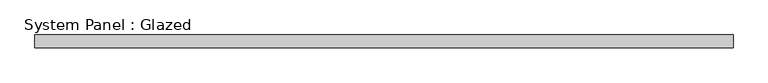
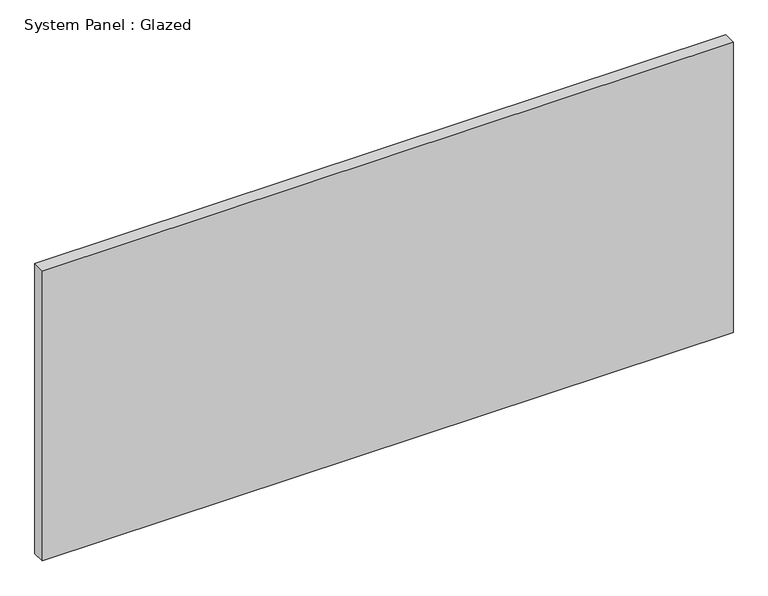
"""IFC4 building model written with IfcOpenShell, lengths in millimetres: plate geometry, System Panel : Glazed."""

from ifc_helpers import new_model, si_unit, origin, origin_with_axes, place, context, project, spatial, polyline, outline, extrude, source, transform, mapped, element, save


def system_panel_glazed_dff4d0e6(model_context):
    return source(origin(), model_context, "Body", "SweptSolid", [
        extrude(outline(polyline([(675.0, -49.5), (-675.0, -49.5), (-675.0, -24.5), (675.0, -24.5), (675.0, -49.5)])), origin_with_axes(), (0.0, 0.0, 1.0), 600.0),
    ])


if __name__ == "__main__":
    model = new_model("IFC4")
    model_context = context("Model", 3, world=origin())
    ifc_project = project(units=[si_unit("LENGTHUNIT", "METRE", prefix="MILLI")], contexts=[model_context])
    site = spatial("IfcSite", under=ifc_project)
    building = spatial("IfcBuilding", under=site)
    placement = place(None, origin())
    system_panel_glazed_shape = system_panel_glazed_dff4d0e6(model_context)
    element("IfcPlate", 1, ObjectType="System Panel : Glazed", at=placement, inside=building, context=model_context, shape_type="MappedRepresentation", body=[
        mapped(system_panel_glazed_shape, transform((0.0, 0.0, 0.0), x_axis=(1.0, 0.0, 0.0), y_axis=(0.0, 1.0, 0.0), z_axis=(0.0, 0.0, 1.0))),
    ])
    save(model, "model.ifc")

# Revit data of these elements
# Type "System Panel : Glazed"
#   Keynote = "H11"
#   Construction Type Id = "GSP4R"
#   Analytic Construction = "1/8 in Pilkington single glazing"
#   Visual Light Transmittance = 0.9
#   Solar Heat Gain Coefficient = 0.86
#   Heat Transfer Coefficient (U) = 6.7069 W/(m²·K)
#   Define Thermal Properties by = 1
# Element 1 (IfcPlate, "System Panel : Glazed")
#   Materials on its faces: "Glass"
# Materials
#   "Glass": class "Glass", colour RGB 0 128 192, transparency 0.9, Description = "Soda Lime Glass", Cost = 0
